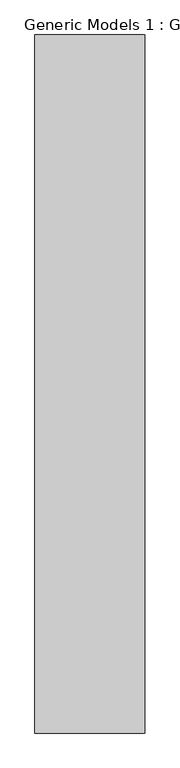
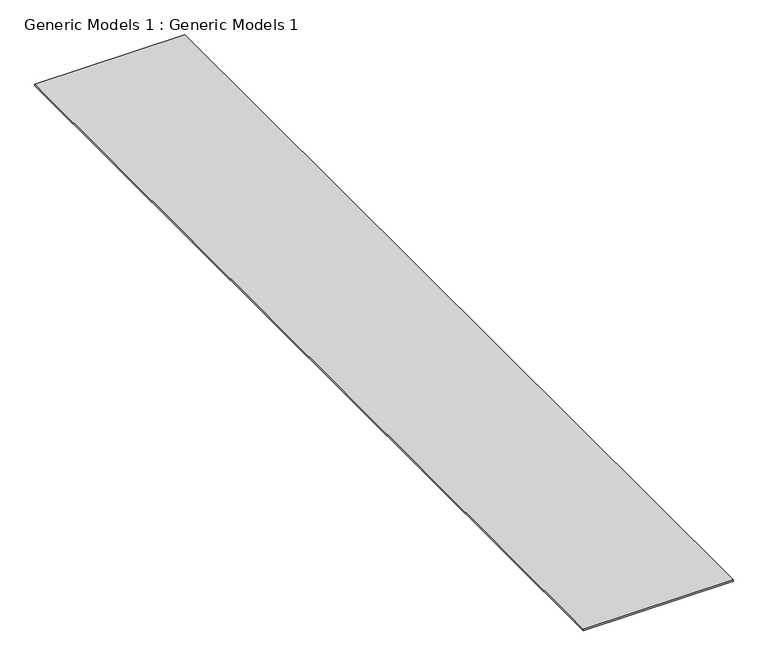
"""IFC4 building model written with IfcOpenShell, lengths in millimetres: proxy geometry, Generic Models 1 : Generic Models 1."""

from ifc_helpers import new_model, si_unit, frame, origin, place, context, project, spatial, polyline, outline, extrude, source, transform, mapped, element, save


def generic_models_1_generic_models_1_344866f9(model_context):
    return source(origin(), model_context, "Body", "SweptSolid", [
        extrude(outline(polyline([(28282.9, 33409.0705427), (28282.9, -23875.569892), (19264.2851519, -23875.569892), (19264.2851519, 33409.0705427), (28282.9, 33409.0705427)])), frame((0.0, 0.0, -76.2), z_axis=(0.0, 0.0, 1.0), x_axis=(1.0, 0.0, 0.0)), (0.0, 0.0, 1.0), 84.2337439),
    ])


if __name__ == "__main__":
    model = new_model("IFC4")
    model_context = context("Model", 3, world=origin())
    ifc_project = project(units=[si_unit("LENGTHUNIT", "METRE", prefix="MILLI")], contexts=[model_context])
    site = spatial("IfcSite", under=ifc_project)
    building = spatial("IfcBuilding", under=site)
    placement = place(None, origin())
    generic_models_1_generic_models_1_shape = generic_models_1_generic_models_1_344866f9(model_context)
    element("IfcBuildingElementProxy", 1, Name="Generic Models 1 : Generic Models 1", ObjectType="Generic Models 1 : Generic Models 1", at=placement, inside=building, context=model_context, shape_type="MappedRepresentation", body=[
        mapped(generic_models_1_generic_models_1_shape, transform((0.0, 0.0, 0.0), x_axis=(1.0, 0.0, 0.0), y_axis=(0.0, 1.0, 0.0), z_axis=(0.0, 0.0, 1.0))),
    ])
    save(model, "model.ifc")
